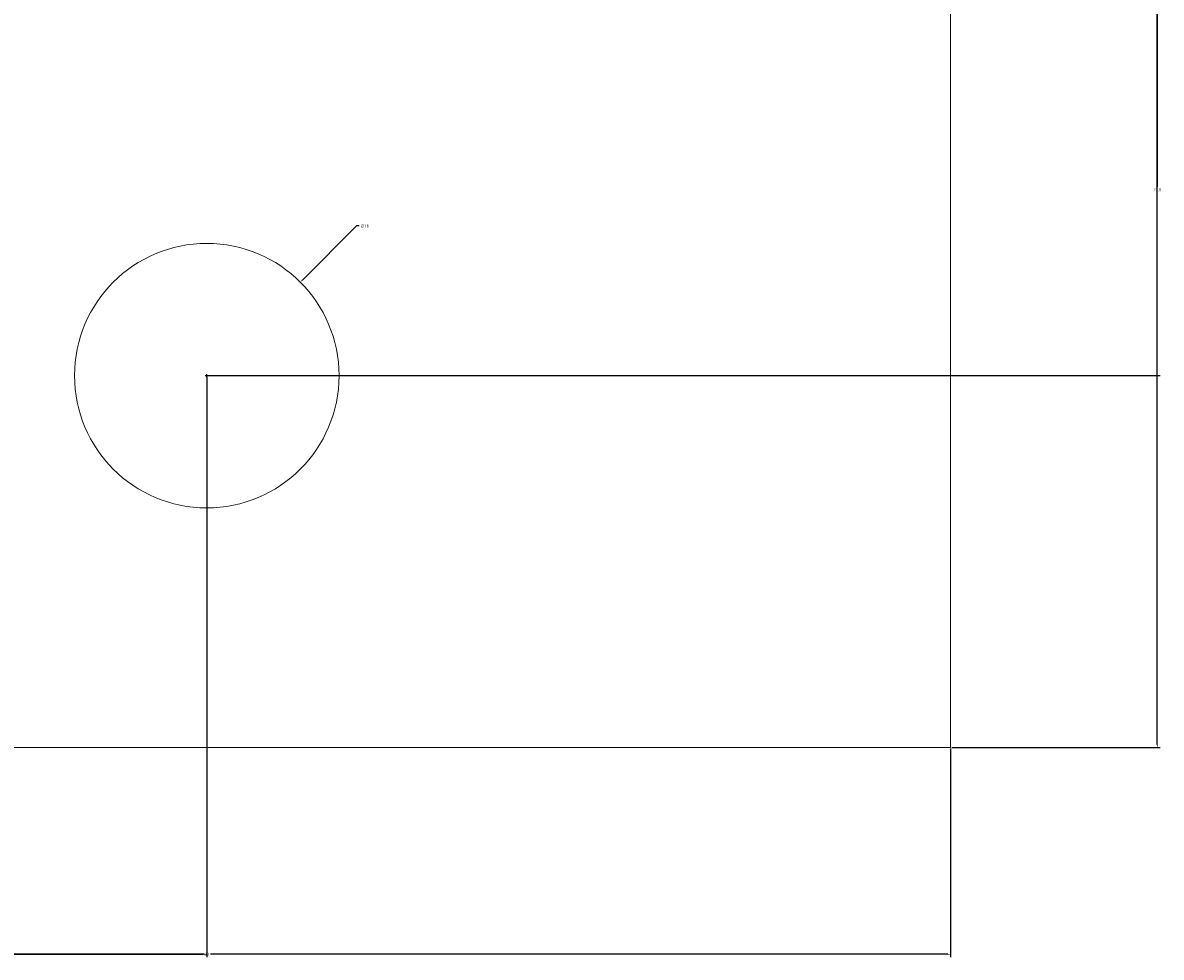
# Model space of a CAD drawing. Units: millimetres. Extents: x 135 to 361, y -58 to 58.
# Tile 4 of 5: x 292 to 361, y -58 to -1. Entities that reach past the tile are written whole.
import ezdxf

# ---------------------------------------------------------------- set-up
doc = ezdxf.new("R2010")
doc.units = ezdxf.units.MM
doc.layers.add('M-CONS', color=8, linetype='Continuous', lineweight=13)
doc.layers.add('M-DIMS', color=2, linetype='Continuous', lineweight=18)
doc.styles.get("Standard").update_dxf_attribs({"font": 'arial.ttf'})
doc.dimstyles.get("Standard").update_dxf_attribs({"dimtxt": 0.18, "dimasz": 0.18, "dimexe": 0.18, "dimexo": 0.0625, "dimgap": 0.09, "dimtad": 0, "dimtih": 1, "dimtoh": 1, "dimdec": 4, "dimzin": 0, "dimdsep": 46, "dimtxsty": 'Standard', "dimcen": 0.09, "dimadec": 0, "dimazin": 0, "dimtfac": 1, "dimtdec": 4, "dimtofl": 0, "dimtmove": 0, "dimatfit": 3, "dimfxl": 1, "dimtolj": 1, "dimtzin": 0, "dimarcsym": 0})

# ---------------------------------------------------------------- blocks, each defined once
blk = doc.blocks.new('*D2')
at = {"layer": 'Defpoints', "color": 0, "transparency": 16777216}
for p in [(347.813, 45), (347.813, -45), (360.313, -45)]:
    blk.add_point(p, dxfattribs=at)
at = {"layer": 'M-DIMS', "color": 0, "lineweight": -2, "transparency": 16777216}
for p, q in [((347.875, 45), (360.493, 45)), ((360.313, 44.82), (360.313, 0.182)), ((360.313, -44.82), (360.313, -0.182)), ((347.875, -45), (360.493, -45))]:
    blk.add_line(p, q, dxfattribs=at)
at = {"layer": 'M-DIMS', "color": 0, "transparency": 16777216}
for points in [[(360.283, 44.82), (360.343, 44.82), (360.313, 45)], [(360.283, -44.82), (360.343, -44.82), (360.313, -45)]]:
    blk.add_solid(points, dxfattribs=at)
at = {"layer": 'M-DIMS', "color": 0, "transparency": 16777216, "insert": (360.313, 0), "char_height": 0.18, "attachment_point": 5}
blk.add_mtext('\\A1;90', dxfattribs=at)
blk = doc.blocks.new('*D6')
at = {"layer": 'Defpoints', "color": 0, "transparency": 16777216}
for p in [(257.813, -45), (347.813, -45), (347.813, -57.5)]:
    blk.add_point(p, dxfattribs=at)
at = {"layer": 'M-DIMS', "color": 0, "lineweight": -2, "transparency": 16777216}
for p, q in [((257.813, -45.062), (257.813, -57.68)), ((347.813, -45.062), (347.813, -57.68)), ((257.993, -57.5), (302.594, -57.5)), ((347.633, -57.5), (303.031, -57.5))]:
    blk.add_line(p, q, dxfattribs=at)
at = {"layer": 'M-DIMS', "color": 0, "transparency": 16777216}
for points in [[(257.993, -57.47), (257.993, -57.53), (257.813, -57.5)], [(347.633, -57.47), (347.633, -57.53), (347.813, -57.5)]]:
    blk.add_solid(points, dxfattribs=at)
at = {"layer": 'M-DIMS', "color": 0, "transparency": 16777216, "insert": (302.813, -57.5), "char_height": 0.18, "attachment_point": 5}
blk.add_mtext('\\A1;90', dxfattribs=at)
blk = doc.blocks.new('*D8')
at = {"layer": 'Defpoints', "color": 0, "transparency": 16777216}
for p in [(302.813, -22.5), (257.813, -45), (302.813, -57.5)]:
    blk.add_point(p, dxfattribs=at)
at = {"layer": 'M-DIMS', "color": 0, "lineweight": -2, "transparency": 16777216}
for p, q in [((302.813, -22.562), (302.813, -57.68)), ((257.813, -45.062), (257.813, -57.68)), ((257.993, -57.5), (280.089, -57.5)), ((302.633, -57.5), (280.536, -57.5))]:
    blk.add_line(p, q, dxfattribs=at)
at = {"layer": 'M-DIMS', "color": 0, "transparency": 16777216}
for points in [[(257.993, -57.47), (257.993, -57.53), (257.813, -57.5)], [(302.633, -57.47), (302.633, -57.53), (302.813, -57.5)]]:
    blk.add_solid(points, dxfattribs=at)
at = {"layer": 'M-DIMS', "color": 0, "transparency": 16777216, "insert": (280.313, -57.5), "char_height": 0.18, "attachment_point": 5}
blk.add_mtext('\\A1;45', dxfattribs=at)
blk = doc.blocks.new('*D9')
at = {"layer": 'Defpoints', "color": 0, "transparency": 16777216}
for p in [(347.813, 0), (360.313, 0), (302.813, -22.5)]:
    blk.add_point(p, dxfattribs=at)
at = {"layer": 'M-DIMS', "color": 0, "lineweight": -2, "transparency": 16777216}
for p, q in [((347.875, 0), (360.493, 0)), ((360.313, -0.18), (360.313, -11.068)), ((360.313, -22.32), (360.313, -11.432)), ((302.875, -22.5), (360.493, -22.5))]:
    blk.add_line(p, q, dxfattribs=at)
at = {"layer": 'M-DIMS', "color": 0, "transparency": 16777216}
for points in [[(360.283, -0.18), (360.343, -0.18), (360.313, 0)], [(360.283, -22.32), (360.343, -22.32), (360.313, -22.5)]]:
    blk.add_solid(points, dxfattribs=at)
at = {"layer": 'M-DIMS', "color": 0, "transparency": 16777216, "insert": (360.313, -11.25), "char_height": 0.18, "attachment_point": 5}
blk.add_mtext('\\A1;22.5', dxfattribs=at)
blk = doc.blocks.new('*D15')
at = {"layer": 'Defpoints', "color": 0, "transparency": 16777216}
for p in [(308.468, -16.842), (297.157, -28.158)]:
    blk.add_point(p, dxfattribs=at)
at = {"layer": 'M-DIMS', "color": 0, "lineweight": -2, "transparency": 16777216}
for p, q in [((311.861, -13.447), (308.595, -16.715)), ((312.041, -13.447), (311.861, -13.447)), ((302.723, -22.5), (302.903, -22.5)), ((302.813, -22.59), (302.813, -22.41))]:
    blk.add_line(p, q, dxfattribs=at)
at = {"layer": 'M-DIMS', "color": 0, "transparency": 16777216}
blk.add_solid([(308.574, -16.693), (308.617, -16.736), (308.468, -16.842)], dxfattribs=at)
at = {"layer": 'M-DIMS', "color": 0, "transparency": 16777216, "insert": (312.358, -13.447), "char_height": 0.18, "attachment_point": 5}
blk.add_mtext('\\A1;∅16', dxfattribs=at)

msp = doc.modelspace()

# ---------------------------------------------------------------- linework, layer by layer
at = {"layer": 'M-CONS', "elevation": 93.744}
msp.add_lwpolyline([(347.813, -45), (257.813, -45), (257.813, 0), (347.813, 0)], close=True, dxfattribs=at)
at = {"layer": 'M-CONS'}
msp.add_circle((302.813, -22.5, 105.744), 8, dxfattribs=at)

# ---------------------------------------------------------------- dimensions: what is measured, and where the dimension line sits
at = {"layer": 'M-DIMS'}
for base, p1, p2, angle, override, picture, middle in [((360.313, -45), (347.813, 45), (347.813, -45), 270, {"dimdec": 0, "dimlfac": 1, "dimrnd": 0, "dimzin": 0, "dimdsep": 46, "dimlunit": 2}, '*D2', (360.313, 0)), ((360.313, 0), (302.813, -22.5), (347.813, 0), 90, {"dimdec": 1, "dimlfac": 1, "dimrnd": 0, "dimzin": 0, "dimdsep": 46, "dimlunit": 2}, '*D9', (360.313, -11.25))]:
    dim = msp.add_linear_dim(base=base, p1=p1, p2=p2, angle=angle, dimstyle='Standard', override=override, dxfattribs=at)
    dim.commit()
    dim.dimension.update_dxf_attribs({"geometry": picture, "text_midpoint": middle})
dim = msp.add_diameter_dim_2p(p1=(297.157, -28.158), p2=(308.468, -16.842), dimstyle='Standard', override={"dimdec": 0, "dimlfac": 1, "dimrnd": 0, "dimzin": 0, "dimdsep": 46, "dimlunit": 2}, dxfattribs=at)
dim.commit()
dim.dimension.update_dxf_attribs({"geometry": '*D15', "text_midpoint": (312.358, -13.447), "dimtype": 163})
for base, p2, picture, middle in [((302.813, -57.5), (302.813, -22.5), '*D8', (280.313, -57.5)), ((347.813, -57.5), (347.813, -45), '*D6', (302.813, -57.5))]:
    dim = msp.add_linear_dim(base=base, p1=(257.813, -45), p2=p2, dimstyle='Standard', override={"dimdec": 0, "dimlfac": 1, "dimrnd": 0, "dimzin": 0, "dimdsep": 46, "dimlunit": 2}, dxfattribs=at)
    dim.commit()
    dim.dimension.update_dxf_attribs({"geometry": picture, "text_midpoint": middle})

doc.saveas('drawing.dxf')
